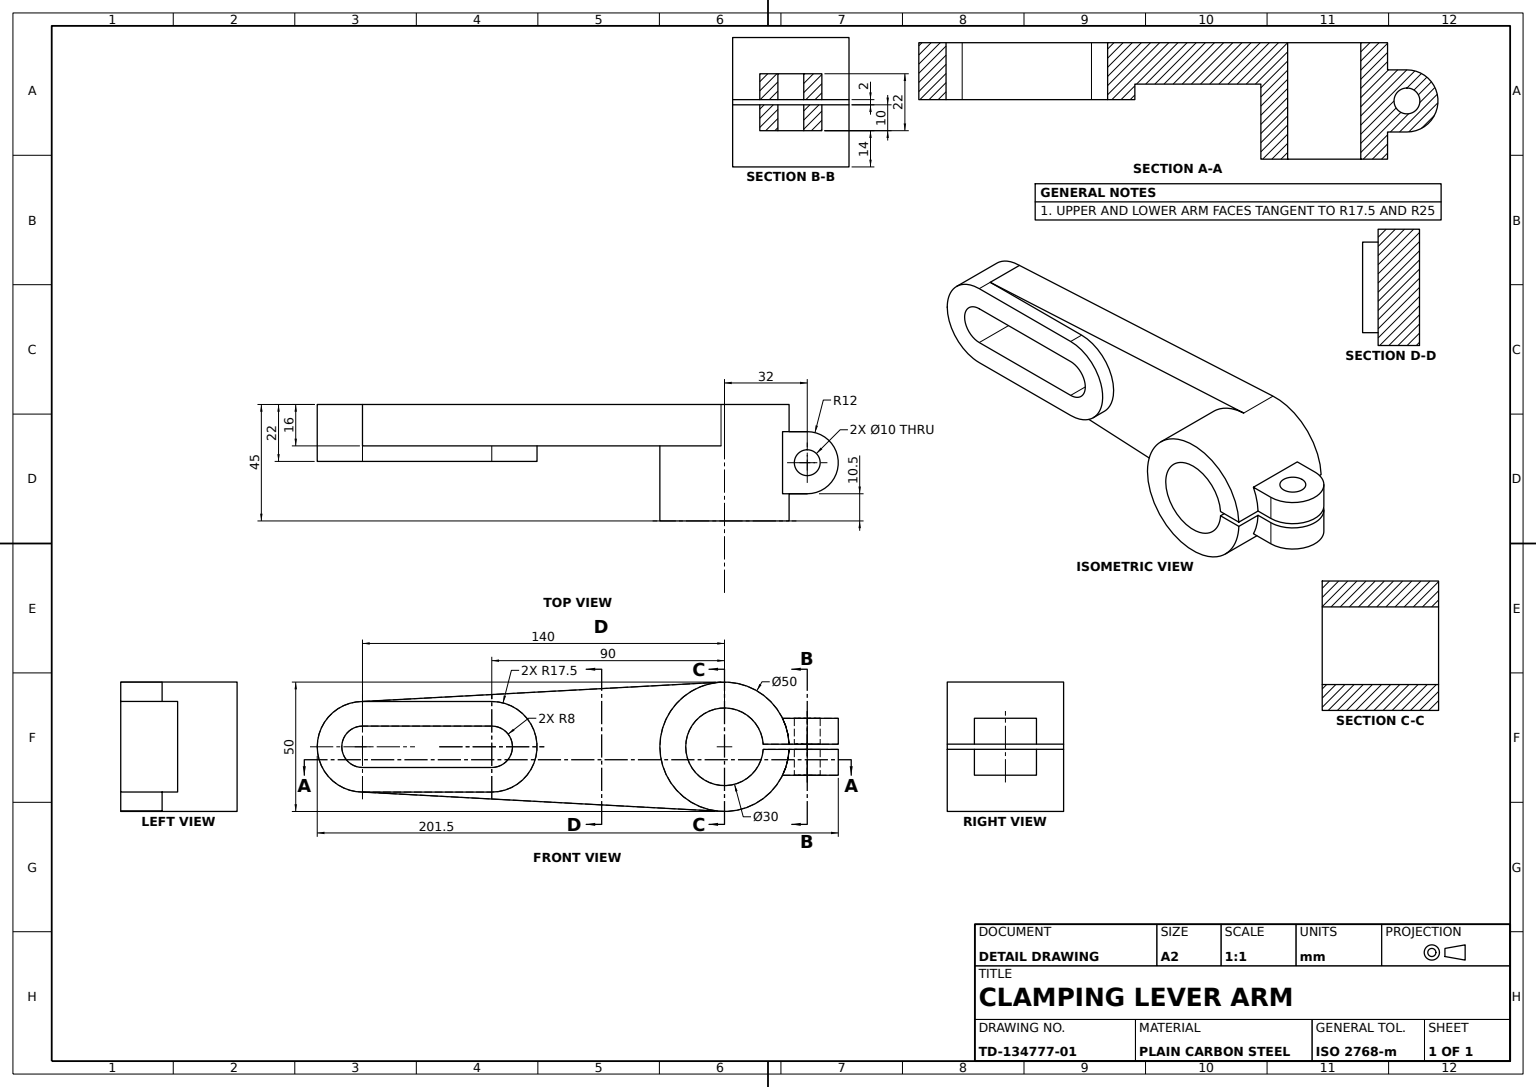
from build123d import *

# Parameters (mm, degrees)
HUB_PROFILE_SKETCH_R       = 25
HUB_PROFILE_SKETCH_R_2     = 15
SHAFT_HUB_50_BORE_30_DEPTH = 45
SLOTTED_ARM_END_DEPTH      = 22
ARM_WEB_DEPTH              = 16
CLAMP_LUG_SKETCH_R         = 5
CLAMP_LUG_DEPTH            = 11
CLAMP_SLIT_1MM_DEPTH       = 166.699275798


with BuildPart() as part:
    # Hub Profile Sketch → Shaft Hub Ø50 Bore Ø30 (new body)
    with BuildSketch(Plane.XY):
        with Locations(Location((0, 0, 0), (0, 0, 180))):
            Circle(HUB_PROFILE_SKETCH_R)
        with Locations(Location((0, 0, 0), (0, 0, 180))):
            Circle(HUB_PROFILE_SKETCH_R_2, mode=Mode.SUBTRACT)
    extrude(amount=SHAFT_HUB_50_BORE_30_DEPTH)



with BuildPart() as body_2:
    # Slotted End Sketch → Slotted Arm End (new body)
    with BuildSketch(Plane.XY):
        with BuildLine():
            Line((-140, 17.5), (-90, 17.5))
            ThreePointArc((-90, 17.5), (-72.5, 0), (-90, -17.5))
            Line((-90, -17.5), (-140, -17.5))
            ThreePointArc((-140, -17.5), (-157.5, 0), (-140, 17.5))
        make_face()
        with BuildLine():
            Line((-140, 8), (-90, 8))
            ThreePointArc((-90, 8), (-82, 0), (-90, -8))
            Line((-90, -8), (-140, -8))
            ThreePointArc((-140, -8), (-148, 0), (-140, 8))
        make_face(mode=Mode.SUBTRACT)
    extrude(amount=SLOTTED_ARM_END_DEPTH)


with BuildPart() as part_1:
    add(part.part)

    add(body_2.part)  # Arm Web merges body 2
    # Arm Web Sketch → Arm Web (add)
    with BuildSketch(Plane.XY):
        with BuildLine():
            Line((-1.3438035, 24.963857718), (-140, 17.5))
            Line((-140, 17.5), (-90, 17.5))
            ThreePointArc((-90, 17.5), (-72.5, 0), (-90, -17.5))
            Line((-90, -17.5), (-140, -17.5))
            Line((-140, -17.5), (-2.6709062, -24.856915739))
            ThreePointArc((-2.6709062, -24.856915739), (-24.991135237, 0.665702292), (-1.3438035, 24.963857718))
        make_face()
    extrude(amount=ARM_WEB_DEPTH)

    # Clamp Lug Sketch → Clamp Lug (add, symmetric)
    with BuildSketch(Plane(origin=(0, 0, 0), x_dir=(1, 0, 0), z_dir=(0, 1, 0))):
        with BuildLine():
            Line((32, -34.5), (25, -34.5))
            Line((25, -34.5), (16.676799829, -34.5))
            Line((16.676799829, -34.5), (16.676799829, -10.5))
            Line((16.676799829, -10.5), (25, -10.5))
            Line((25, -10.5), (32, -10.5))
            ThreePointArc((32, -10.5), (44, -22.5), (32, -34.5))
        make_face()
        with Locations(Location((32, -22.5, 0), (0, 0, 270))):
            Circle(CLAMP_LUG_SKETCH_R, mode=Mode.SUBTRACT)
    extrude(amount=CLAMP_LUG_DEPTH, both=True)

    # Clamp Slit Sketch → Clamp Slit 1mm (cut, through all)
    with BuildSketch(Plane.XY.offset(45)):
        with BuildLine():
            Line((14.966629547, -1), (44, -1))
            Line((44, -1), (47.131344101, -1))
            Line((47.131344101, -1), (47.131344101, 1))
            Line((47.131344101, 1), (43.927311634, 1))
            Line((43.927311634, 1), (14.966629547, 1))
            ThreePointArc((14.966629547, 1), (15, 0), (14.966629547, -1))
        make_face()
    extrude(amount=-CLAMP_SLIT_1MM_DEPTH, mode=Mode.SUBTRACT)


solid = part_1.part
